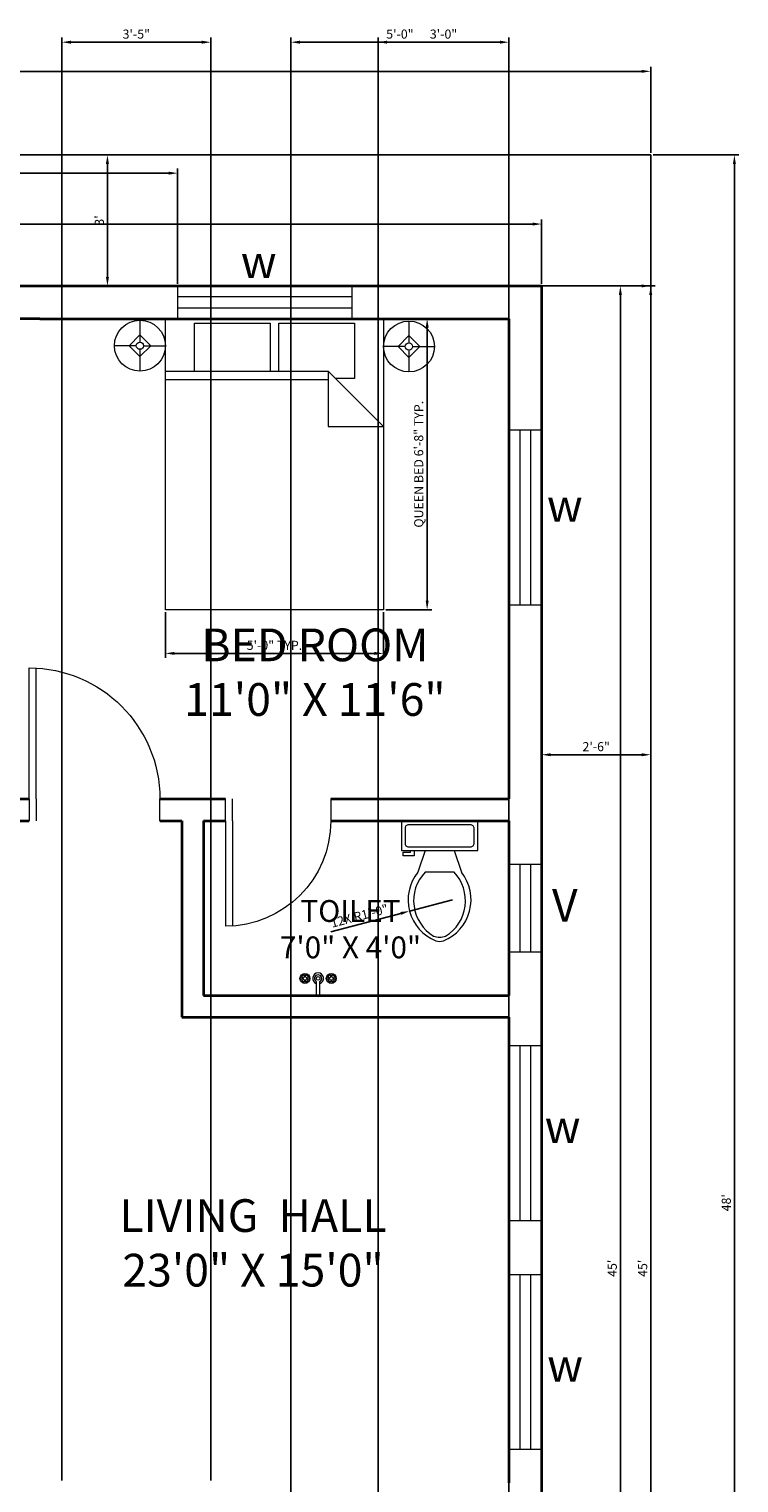
# Model space of a CAD drawing. Units: inches. Extents: x 2009 to 2890, y 2827 to 3504.
# Tile 3 of 6: x 2235 to 2430, y 3105 to 3504. Entities that reach past the tile are written whole.
import ezdxf

# ---------------------------------------------------------------- set-up
doc = ezdxf.new("R2010")
doc.units = ezdxf.units.IN
for name, color, linetype, lineweight in [('A-ANNO-DIMS', 2, 'Continuous', 18), ('A-ANNO-TEXT', 3, 'Continuous', 18), ('A-AREA-IDEN', 7, 'Continuous', 25), ('A-DOOR', 3, 'Continuous', 18), ('A-FLOR-FIXT', 9, 'Continuous', 18), ('A-FURN', 8, 'Continuous', 18), ('A-GLAZ', 4, 'Continuous', 18), ('A-WALL', 7, 'Continuous', 35), ('C-PROP', 8, 'Continuous', 25)]:
    doc.layers.add(name, color=color, linetype=linetype, lineweight=lineweight)
doc.styles.get("Standard").update_dxf_attribs({"font": 'arial.ttf'})
doc.dimstyles.new('ISO-25', dxfattribs={"dimtxt": 2.5, "dimasz": 2.5, "dimexe": 1.25, "dimexo": 0.625, "dimtad": 1, "dimdec": 0, "dimlunit": 3, "dimtxsty": 'Standard', "dimcen": 2.5, "dimadec": 0, "dimazin": 0, "dimtfac": 1, "dimtdec": 0, "dimtmove": 0, "dimatfit": 3, "dimfxl": 1, "dimarcsym": 0})

# ---------------------------------------------------------------- blocks, each defined once
blk = doc.blocks.new('Bed - Queen')
for p, q in [((0, -80.00003), (0, 0)), ((0, 0), (59.99999, 0)), ((59.99999, 0), (59.99999, -80.00003)), ((7.99999, -1.2), (28.79998, -1.2)), ((7.99999, -14.4), (7.99999, -1.2)), ((28.79998, -1.2), (28.79998, -14.4)), ((31.19999, -1.2), (51.99999, -1.2)), ((31.19999, -14.4), (31.19999, -1.2)), ((51.99999, -1.2), (51.99999, -16.4)), ((0, -14.4), (44.8, -14.4)), ((59.99999, -29.6), (44.8, -14.4)), ((44.8, -14.4), (44.8, -29.6)), ((44.8, -16.8), (0, -16.8)), ((51.99999, -16.4), (46.79936, -16.4)), ((44.8, -29.6), (59.99999, -29.6)), ((59.99999, -80.00003), (0, -80.00003))]:
    blk.add_line(p, q)
blk = doc.blocks.new('Lamp - Table')
for p, q in [((0, 7), (0, 1)), ((-1, 0), (-7, 0)), ((0, 3), (-3, 0)), ((-3, 0), (0, -3)), ((3, 0), (0, 3)), ((0, -3), (3, 0)), ((1, 0), (7, 0)), ((0, -1), (0, -7))]:
    blk.add_line(p, q)
for radius in [7, 1]:
    blk.add_circle((0, 0), radius)
blk = doc.blocks.new('Toilet - top')
for p, q in [((9.5, -6), (9.5, -2)), ((-10, -8.5), (-8, -8.5)), ((-10, -9.5), (-10, -8.5)), ((-7, -9.5), (-10, -9.5)), ((-8, -8.5), (-8, -8)), ((-7, -8), (-7, -9.5)), ((-4, -8), (-6, -14)), ((4, -8), (6, -14)), ((4, -14), (-4, -14))]:
    blk.add_line(p, q)
blk.add_lwpolyline([(10.5, -8), (10.5, 0), (-10.5, 0), (-10.5, -8)], close=True)
for points in [[(-9.5, -2), (-9.5, -6)], [(8.5, -1), (-8.5, -1)], [(-8.5, -7), (8.5, -7)]]:
    blk.add_lwpolyline(points)
for centre, radius, start, end in [((-8.62, -1.88), 0.884, 81.8699, 188.1301), ((8.62, -1.88), 0.884, 351.8699, 98.1301), ((-8.62, -6.12), 0.884, 171.8699, 278.1301), ((8.62, -6.12), 0.884, 261.8699, 8.1301), ((3.52, -21.58), 12.17, 141.4691, 247.9714), ((4.2, -21.82), 11.33, 136.3677, 238.9468), ((-3.52, -21.58), 12.17, 292.0284, 38.5307), ((-4.2, -21.82), 11.33, 301.053, 43.6321), ((0, -27.88), 4, 245.7318, 294.2682), ((0, -29), 4, 254.8605, 285.1395)]:
    blk.add_arc(centre, radius, start, end)
blk = doc.blocks.new('*D8')
at = {"layer": 'A-ANNO-DIMS', "color": 0, "lineweight": -2, "transparency": 16777216}
for p, q in [((2075.76, 3434.16), (2075.76, 3451.81)), ((2078.26, 3450.56), (2373.26, 3450.56)), ((2375.76, 3434.16), (2375.76, 3451.81))]:
    blk.add_line(p, q, dxfattribs=at)
at = {"layer": 'A-ANNO-DIMS', "color": 0, "transparency": 16777216}
for points in [[(2078.26, 3450.97), (2078.26, 3450.14), (2075.76, 3450.56)], [(2373.26, 3450.97), (2373.26, 3450.14), (2375.76, 3450.56)]]:
    blk.add_solid(points, dxfattribs=at)
at = {"layer": 'Defpoints', "color": 0, "transparency": 16777216}
for p in [(2375.76, 3450.56), (2075.76, 3433.54), (2375.76, 3433.54)]:
    blk.add_point(p, dxfattribs=at)
at = {"layer": 'A-ANNO-DIMS', "color": 0, "transparency": 16777216, "insert": (2225.76, 3452.46), "char_height": 2.5, "attachment_point": 5}
blk.add_mtext("25'", dxfattribs=at)
blk = doc.blocks.new('*D9')
at = {"layer": 'A-ANNO-DIMS', "color": 0, "lineweight": -2, "transparency": 16777216}
for p, q in [((2376.39, 3433.54), (2398.66, 3433.54)), ((2397.41, 3431.04), (2397.41, 2896.04)), ((2376.39, 2893.54), (2398.66, 2893.54))]:
    blk.add_line(p, q, dxfattribs=at)
at = {"layer": 'A-ANNO-DIMS', "color": 0, "transparency": 16777216}
for points in [[(2396.99, 3431.04), (2397.83, 3431.04), (2397.41, 3433.54)], [(2396.99, 2896.04), (2397.83, 2896.04), (2397.41, 2893.54)]]:
    blk.add_solid(points, dxfattribs=at)
at = {"layer": 'Defpoints', "color": 0, "transparency": 16777216}
for p in [(2375.76, 3433.54), (2375.76, 2893.54), (2397.41, 2893.54)]:
    blk.add_point(p, dxfattribs=at)
at = {"layer": 'A-ANNO-DIMS', "color": 0, "transparency": 16777216, "insert": (2395.51, 3163.54), "char_height": 2.5, "attachment_point": 5, "rotation": 90}
blk.add_mtext("45'", dxfattribs=at)
blk = doc.blocks.new('*D10')
at = {"layer": 'A-ANNO-DIMS', "color": 0, "lineweight": -2, "transparency": 16777216}
for p, q in [((2045.76, 3470.16), (2045.76, 3493.78)), ((2405.76, 3470.16), (2405.76, 3493.78)), ((2048.26, 3492.53), (2403.26, 3492.53))]:
    blk.add_line(p, q, dxfattribs=at)
at = {"layer": 'A-ANNO-DIMS', "color": 0, "transparency": 16777216}
for points in [[(2048.26, 3492.95), (2048.26, 3492.11), (2045.76, 3492.53)], [(2403.26, 3492.95), (2403.26, 3492.11), (2405.76, 3492.53)]]:
    blk.add_solid(points, dxfattribs=at)
at = {"layer": 'Defpoints', "color": 0, "transparency": 16777216}
for p in [(2405.76, 3492.53), (2045.76, 3469.54), (2405.76, 3469.54)]:
    blk.add_point(p, dxfattribs=at)
at = {"layer": 'A-ANNO-DIMS', "color": 0, "transparency": 16777216, "insert": (2225.76, 3494.43), "char_height": 2.5, "attachment_point": 5}
blk.add_mtext("30'", dxfattribs=at)
blk = doc.blocks.new('*D11')
at = {"layer": 'A-ANNO-DIMS', "color": 0, "lineweight": -2, "transparency": 16777216}
for p, q in [((2406.39, 3469.54), (2430.02, 3469.54)), ((2428.77, 3467.04), (2428.77, 2896.04)), ((2406.39, 2893.54), (2430.02, 2893.54))]:
    blk.add_line(p, q, dxfattribs=at)
at = {"layer": 'A-ANNO-DIMS', "color": 0, "transparency": 16777216}
for points in [[(2428.36, 3467.04), (2429.19, 3467.04), (2428.77, 3469.54)], [(2428.36, 2896.04), (2429.19, 2896.04), (2428.77, 2893.54)]]:
    blk.add_solid(points, dxfattribs=at)
at = {"layer": 'Defpoints', "color": 0, "transparency": 16777216}
for p in [(2405.76, 3469.54), (2405.76, 2893.54), (2428.77, 2893.54)]:
    blk.add_point(p, dxfattribs=at)
at = {"layer": 'A-ANNO-DIMS', "color": 0, "transparency": 16777216, "insert": (2426.87, 3181.54), "char_height": 2.5, "attachment_point": 5, "rotation": 90}
blk.add_mtext("48'", dxfattribs=at)
blk = doc.blocks.new('Faucet - Bathroom top')
for p, q in [((-4.107, 0.125), (-4.375, 0.125)), ((-3.75, 0.4788), (-3.75, 0.75)), ((-3.5, 0.482), (-3.5, 0.75)), ((-3.1461, 0.125), (-2.875, 0.125)), ((3.143, 0.125), (2.875, 0.125)), ((3.5, 0.4788), (3.5, 0.75)), ((3.75, 0.482), (3.75, 0.75)), ((4.1039, 0.125), (4.375, 0.125)), ((-4.1039, -0.125), (-4.375, -0.125)), ((-3.75, -0.4821), (-3.75, -0.75)), ((-3.5, -0.4789), (-3.5, -0.75)), ((-3.143, -0.125), (-2.875, -0.125)), ((-0.5, -0.8639), (-0.5, -4.5)), ((0.5, -4.5), (0.5, -0.8631)), ((3.1461, -0.125), (2.875, -0.125)), ((3.5, -0.4821), (3.5, -0.75)), ((3.75, -0.4789), (3.75, -0.75)), ((4.107, -0.125), (4.375, -0.125))]:
    blk.add_line(p, q)
for centre, radius in [((-3.625, 0), 1.375), ((-4.625, 0), 0.2795), ((-3.625, 0), 0.5), ((-3.625, 1), 0.2795), ((-2.625, 0), 0.2795), ((0, 0), 0.5), ((3.625, 0), 1.375), ((2.625, 0), 0.2795), ((3.625, 0), 0.5), ((3.625, 1), 0.2795), ((4.625, 0), 0.2795), ((-3.625, -1), 0.2795), ((3.625, -1), 0.2795)]:
    blk.add_circle(centre, radius)
for centre, radius, start, end in [((-3.625, 0), 1, 105.2407, 164.2093), ((-3.625, 0), 1, 16.44125, 74.07887), ((0, 0), 1.5, 289.6514, 250.3603), ((0, 0), 1, 300.3431, 239.7554), ((3.625, 0), 1, 106.12, 164.0884), ((3.625, 0), 1, 16.23422, 73.90469), ((-3.625, 0), 1, 196.2342, 253.9047), ((-3.625, 0), 1, 286.12, 344.0884), ((3.625, 0), 1, 196.4413, 254.0789), ((3.625, 0), 1, 285.2407, 344.2093), ((0, -4.5), 0.5, 180, 0)]:
    blk.add_arc(centre, radius, start, end)
blk = doc.blocks.new('*D16')
at = {"layer": 'A-ANNO-DIMS', "color": 0, "lineweight": -2, "transparency": 16777216}
for p, q in [((2045.76, 3468.91), (2045.76, 3432.29)), ((2405.76, 3468.91), (2405.76, 3432.29)), ((2403.26, 3433.54), (2048.26, 3433.54))]:
    blk.add_line(p, q, dxfattribs=at)
at = {"layer": 'A-ANNO-DIMS', "color": 0, "transparency": 16777216}
for points in [[(2048.26, 3433.96), (2048.26, 3433.12), (2045.76, 3433.54)], [(2403.26, 3433.96), (2403.26, 3433.12), (2405.76, 3433.54)]]:
    blk.add_solid(points, dxfattribs=at)
at = {"layer": 'Defpoints', "color": 0, "transparency": 16777216}
for p in [(2045.76, 3469.54), (2405.76, 3469.54), (2045.76, 3433.54)]:
    blk.add_point(p, dxfattribs=at)
at = {"layer": 'A-ANNO-DIMS', "color": 0, "transparency": 16777216, "insert": (2225.76, 3435.44), "char_height": 2.5, "attachment_point": 5}
blk.add_mtext("30'", dxfattribs=at)
blk = doc.blocks.new('*D17')
at = {"layer": 'A-ANNO-DIMS', "color": 0, "lineweight": -2, "transparency": 16777216}
for p, q in [((2257.96, 3469.54), (2255.07, 3469.54)), ((2256.32, 3467.04), (2256.32, 3436.04)), ((2257.96, 3433.54), (2255.07, 3433.54))]:
    blk.add_line(p, q, dxfattribs=at)
at = {"layer": 'A-ANNO-DIMS', "color": 0, "transparency": 16777216}
for points in [[(2255.9, 3467.04), (2256.74, 3467.04), (2256.32, 3469.54)], [(2255.9, 3436.04), (2256.74, 3436.04), (2256.32, 3433.54)]]:
    blk.add_solid(points, dxfattribs=at)
at = {"layer": 'Defpoints', "color": 0, "transparency": 16777216}
for p in [(2258.58, 3469.54), (2256.32, 3433.54), (2258.58, 3433.54)]:
    blk.add_point(p, dxfattribs=at)
at = {"layer": 'A-ANNO-DIMS', "color": 0, "transparency": 16777216, "insert": (2254.42, 3451.54), "char_height": 2.5, "attachment_point": 5, "rotation": 90}
blk.add_mtext("3'", dxfattribs=at)
blk = doc.blocks.new('*D18')
at = {"layer": 'A-ANNO-DIMS', "color": 0, "lineweight": -2, "transparency": 16777216}
for p, q in [((2376.39, 3433.54), (2407.01, 3433.54)), ((2405.76, 3431.04), (2405.76, 2896.04)), ((2376.39, 2893.54), (2407.01, 2893.54))]:
    blk.add_line(p, q, dxfattribs=at)
at = {"layer": 'A-ANNO-DIMS', "color": 0, "transparency": 16777216}
for points in [[(2405.35, 3431.04), (2406.18, 3431.04), (2405.76, 3433.54)], [(2405.35, 2896.04), (2406.18, 2896.04), (2405.76, 2893.54)]]:
    blk.add_solid(points, dxfattribs=at)
at = {"layer": 'Defpoints', "color": 0, "transparency": 16777216}
for p in [(2375.76, 3433.54), (2375.76, 2893.54), (2405.76, 2893.54)]:
    blk.add_point(p, dxfattribs=at)
at = {"layer": 'A-ANNO-DIMS', "color": 0, "transparency": 16777216, "insert": (2403.87, 3163.54), "char_height": 2.5, "attachment_point": 5, "rotation": 90}
blk.add_mtext("45'", dxfattribs=at)
blk = doc.blocks.new('*D19')
at = {"layer": 'A-ANNO-DIMS', "color": 0, "lineweight": -2, "transparency": 16777216}
for p, q in [((2376.39, 3433.54), (2407.01, 3433.54)), ((2405.76, 3431.04), (2405.76, 2896.04)), ((2376.39, 2893.54), (2407.01, 2893.54))]:
    blk.add_line(p, q, dxfattribs=at)
at = {"layer": 'A-ANNO-DIMS', "color": 0, "transparency": 16777216}
for points in [[(2405.35, 3431.04), (2406.18, 3431.04), (2405.76, 3433.54)], [(2405.35, 2896.04), (2406.18, 2896.04), (2405.76, 2893.54)]]:
    blk.add_solid(points, dxfattribs=at)
at = {"layer": 'Defpoints', "color": 0, "transparency": 16777216}
for p in [(2375.76, 3433.54), (2375.76, 2893.54), (2405.76, 2893.54)]:
    blk.add_point(p, dxfattribs=at)
at = {"layer": 'A-ANNO-DIMS', "color": 0, "transparency": 16777216, "insert": (2403.87, 3163.54), "char_height": 2.5, "attachment_point": 5, "rotation": 90}
blk.add_mtext("45'", dxfattribs=at)
blk = doc.blocks.new('*D20')
at = {"layer": 'A-ANNO-DIMS', "color": 0, "lineweight": -2, "transparency": 16777216}
for p, q in [((2375.76, 3320.11), (2375.76, 3303.44)), ((2405.76, 3320.11), (2405.76, 3303.44)), ((2378.26, 3304.69), (2403.26, 3304.69))]:
    blk.add_line(p, q, dxfattribs=at)
at = {"layer": 'A-ANNO-DIMS', "color": 0, "transparency": 16777216}
for points in [[(2378.26, 3305.11), (2378.26, 3304.27), (2375.76, 3304.69)], [(2403.26, 3305.11), (2403.26, 3304.27), (2405.76, 3304.69)]]:
    blk.add_solid(points, dxfattribs=at)
at = {"layer": 'Defpoints', "color": 0, "transparency": 16777216}
for p in [(2375.76, 3320.74), (2405.76, 3320.74), (2405.76, 3304.69)]:
    blk.add_point(p, dxfattribs=at)
at = {"layer": 'A-ANNO-DIMS', "color": 0, "transparency": 16777216, "insert": (2390.76, 3306.59), "char_height": 2.5, "attachment_point": 5}
blk.add_mtext('2\'-6"', dxfattribs=at)
blk = doc.blocks.new('WIN-48IN')
for p, q in [((0, 48), (0, 0)), ((9, 48), (0, 48)), ((3, 48), (3, 0)), ((6, 0), (6, 48)), ((9, 0), (9, 48)), ((0, 0), (9, 0))]:
    blk.add_line(p, q)
blk = doc.blocks.new('VENT-24IN')
for p, q in [((0, 24), (0, 0)), ((9, 24), (0, 24)), ((3, 24), (3, 0)), ((6, 0), (6, 24)), ((9, 0), (9, 24)), ((0, 0), (9, 0))]:
    blk.add_line(p, q)
blk = doc.blocks.new('DOOR-29IN')
for p, q in [((0, 35), (0, 29)), ((27, 29), (27, 35)), ((29, 29), (29, 35)), ((27, 29), (27, 0)), ((29, 29), (29, 0))]:
    blk.add_line(p, q)
blk.add_arc((29, 29), 29, 180, 270)
blk = doc.blocks.new('DOOR-36IN')
for p, q in [((34, 6), (34, 42)), ((36, 6), (36, 42)), ((0, 0), (0, 6)), ((34, 6), (34, 0)), ((36, 6), (36, 0))]:
    blk.add_line(p, q)
blk.add_arc((36, 6), 36, 90, 180)
blk = doc.blocks.new('*D43')
at = {"layer": 'A-ANNO-DIMS', "color": 0, "lineweight": -2, "transparency": 16777216}
for p, q in [((2332.89, 3424.54), (2345.51, 3424.54)), ((2344.26, 3347.04), (2344.26, 3422.04)), ((2332.89, 3344.54), (2345.51, 3344.54))]:
    blk.add_line(p, q, dxfattribs=at)
at = {"layer": 'A-ANNO-DIMS', "color": 0, "transparency": 16777216}
for points in [[(2343.85, 3422.04), (2344.68, 3422.04), (2344.26, 3424.54)], [(2343.85, 3347.04), (2344.68, 3347.04), (2344.26, 3344.54)]]:
    blk.add_solid(points, dxfattribs=at)
at = {"layer": 'Defpoints', "color": 0, "transparency": 16777216}
for p in [(2332.26, 3424.54), (2344.26, 3424.54), (2332.26, 3344.54)]:
    blk.add_point(p, dxfattribs=at)
at = {"layer": 'A-ANNO-DIMS', "color": 0, "transparency": 16777216, "insert": (2342.27, 3384.54), "char_height": 2.5, "attachment_point": 5, "rotation": 90}
blk.add_mtext('QUEEN BED 6\'-8" TYP.', dxfattribs=at)
blk = doc.blocks.new('*D44')
at = {"layer": 'A-ANNO-DIMS', "color": 0, "lineweight": -2, "transparency": 16777216}
for p, q in [((2272.26, 3343.91), (2272.26, 3331.29)), ((2332.26, 3343.91), (2332.26, 3331.29)), ((2274.76, 3332.54), (2329.76, 3332.54))]:
    blk.add_line(p, q, dxfattribs=at)
at = {"layer": 'A-ANNO-DIMS', "color": 0, "transparency": 16777216}
for points in [[(2274.76, 3332.96), (2274.76, 3332.12), (2272.26, 3332.54)], [(2329.76, 3332.96), (2329.76, 3332.12), (2332.26, 3332.54)]]:
    blk.add_solid(points, dxfattribs=at)
at = {"layer": 'Defpoints', "color": 0, "transparency": 16777216}
for p in [(2272.26, 3344.54), (2332.26, 3344.54), (2332.26, 3332.54)]:
    blk.add_point(p, dxfattribs=at)
at = {"layer": 'A-ANNO-DIMS', "color": 0, "transparency": 16777216, "insert": (2302.26, 3334.44), "char_height": 2.5, "attachment_point": 5}
blk.add_mtext('5\'-0" TYP.', dxfattribs=at)
blk = doc.blocks.new('*D66')
at = {"layer": 'A-ANNO-DIMS', "color": 0, "lineweight": -2, "transparency": 16777216}
for p, q in [((2330.76, 3011.16), (2330.76, 3501.79)), ((2366.76, 3011.16), (2366.76, 3501.79)), ((2333.26, 3500.54), (2364.26, 3500.54))]:
    blk.add_line(p, q, dxfattribs=at)
at = {"layer": 'A-ANNO-DIMS', "color": 0, "transparency": 16777216}
for points in [[(2333.26, 3500.96), (2333.26, 3500.12), (2330.76, 3500.54)], [(2364.26, 3500.96), (2364.26, 3500.12), (2366.76, 3500.54)]]:
    blk.add_solid(points, dxfattribs=at)
at = {"layer": 'Defpoints', "color": 0, "transparency": 16777216}
for p in [(2366.76, 3500.54), (2330.76, 3010.54), (2366.76, 3010.54)]:
    blk.add_point(p, dxfattribs=at)
at = {"layer": 'A-ANNO-DIMS', "color": 0, "transparency": 16777216, "insert": (2348.76, 3502.44), "char_height": 2.5, "attachment_point": 5}
blk.add_mtext('3\'-0"', dxfattribs=at)
blk = doc.blocks.new('*D68')
at = {"layer": 'A-ANNO-DIMS', "color": 0, "lineweight": -2, "transparency": 16777216}
for p, q in [((2306.76, 3048.16), (2306.76, 3501.79)), ((2366.76, 3048.16), (2366.76, 3501.79)), ((2309.26, 3500.54), (2364.26, 3500.54))]:
    blk.add_line(p, q, dxfattribs=at)
at = {"layer": 'A-ANNO-DIMS', "color": 0, "transparency": 16777216}
for points in [[(2309.26, 3500.96), (2309.26, 3500.12), (2306.76, 3500.54)], [(2364.26, 3500.96), (2364.26, 3500.12), (2366.76, 3500.54)]]:
    blk.add_solid(points, dxfattribs=at)
at = {"layer": 'Defpoints', "color": 0, "transparency": 16777216}
for p in [(2366.76, 3500.54), (2306.76, 3047.54), (2366.76, 3047.54)]:
    blk.add_point(p, dxfattribs=at)
at = {"layer": 'A-ANNO-DIMS', "color": 0, "transparency": 16777216, "insert": (2336.76, 3502.44), "char_height": 2.5, "attachment_point": 5}
blk.add_mtext('5\'-0"', dxfattribs=at)
blk = doc.blocks.new('*D75')
at = {"layer": 'A-ANNO-DIMS', "color": 0, "lineweight": -2, "transparency": 16777216}
for p, q in [((2243.76, 3105.16), (2243.76, 3501.79)), ((2284.76, 3105.16), (2284.76, 3501.79)), ((2246.26, 3500.54), (2282.26, 3500.54))]:
    blk.add_line(p, q, dxfattribs=at)
at = {"layer": 'A-ANNO-DIMS', "color": 0, "transparency": 16777216}
for points in [[(2246.26, 3500.96), (2246.26, 3500.12), (2243.76, 3500.54)], [(2282.26, 3500.96), (2282.26, 3500.12), (2284.76, 3500.54)]]:
    blk.add_solid(points, dxfattribs=at)
at = {"layer": 'Defpoints', "color": 0, "transparency": 16777216}
for p in [(2284.76, 3500.54), (2243.76, 3104.54), (2284.76, 3104.54)]:
    blk.add_point(p, dxfattribs=at)
at = {"layer": 'A-ANNO-DIMS', "color": 0, "transparency": 16777216, "insert": (2264.26, 3502.44), "char_height": 2.5, "attachment_point": 5}
blk.add_mtext('3\'-5"', dxfattribs=at)
blk = doc.blocks.new('*D77')
at = {"layer": 'A-ANNO-DIMS', "color": 0, "lineweight": -2, "transparency": 16777216}
for p, q in [((2130.69, 3434.16), (2130.69, 3465.79)), ((2275.62, 3434.16), (2275.62, 3465.79)), ((2133.19, 3464.54), (2273.12, 3464.54))]:
    blk.add_line(p, q, dxfattribs=at)
at = {"layer": 'A-ANNO-DIMS', "color": 0, "transparency": 16777216}
for points in [[(2133.19, 3464.96), (2133.19, 3464.12), (2130.69, 3464.54)], [(2273.12, 3464.96), (2273.12, 3464.12), (2275.62, 3464.54)]]:
    blk.add_solid(points, dxfattribs=at)
at = {"layer": 'Defpoints', "color": 0, "transparency": 16777216}
for p in [(2275.62, 3464.54), (2130.69, 3433.54), (2275.62, 3433.54)]:
    blk.add_point(p, dxfattribs=at)
at = {"layer": 'A-ANNO-DIMS', "color": 0, "transparency": 16777216, "insert": (2203.16, 3466.42), "char_height": 2.5, "attachment_point": 5}
blk.add_mtext('12\'-1"', dxfattribs=at)
blk = doc.blocks.new('*D91')
at = {"layer": 'A-ANNO-DIMS', "color": 0, "lineweight": -2, "transparency": 16777216}
for p, q in [((2351.2, 3264.81), (2339.43, 3261.71)), ((2317.8, 3256.03), (2337.01, 3261.08))]:
    blk.add_line(p, q, dxfattribs=at)
at = {"layer": 'A-ANNO-DIMS', "color": 0, "transparency": 16777216}
blk.add_solid([(2336.91, 3261.48), (2337.12, 3260.68), (2339.43, 3261.71)], dxfattribs=at)
at = {"layer": 'Defpoints', "color": 0, "transparency": 16777216}
for p in [(2351.2, 3264.81), (2339.43, 3261.71)]:
    blk.add_point(p, dxfattribs=at)
at = {"layer": 'A-ANNO-DIMS', "color": 0, "transparency": 16777216, "insert": (2325.71, 3260.08), "char_height": 2.5, "attachment_point": 5, "rotation": 14.7219}
blk.add_mtext('12X R1\'-0"', dxfattribs=at)

msp = doc.modelspace()

# ---------------------------------------------------------------- linework, layer by layer
at = {"layer": 'A-WALL'}
for p, q in [((2075.76, 3433.54), (2375.76, 3433.54)), ((2375.76, 3433.54), (2375.76, 2893.54)), ((2237.76, 3424.54), (2228.76, 3424.54)), ((2237.76, 3424.54), (2366.76, 3424.54)), ((2366.76, 3424.54), (2366.76, 3292.54)), ((2228.76, 3292.54), (2234.76, 3292.54)), ((2228.76, 3292.54), (2234.76, 3292.54)), ((2270.76, 3292.54), (2288.76, 3292.54)), ((2317.76, 3292.54), (2366.76, 3292.54)), ((2216.76, 3286.54), (2234.76, 3286.54)), ((2270.76, 3286.54), (2276.76, 3286.54)), ((2276.76, 3286.54), (2276.76, 3238.54)), ((2282.76, 3286.54), (2282.76, 3238.54)), ((2282.76, 3286.54), (2288.76, 3286.54)), ((2282.76, 3286.54), (2288.76, 3286.54)), ((2317.76, 3286.54), (2366.76, 3286.54)), ((2366.76, 3286.54), (2366.76, 3238.54)), ((2276.76, 3238.54), (2276.76, 3232.54)), ((2282.76, 3238.54), (2366.76, 3238.54)), ((2276.76, 3232.54), (2366.76, 3232.54)), ((2366.76, 3232.54), (2366.76, 3104.54))]:
    msp.add_line(p, q, dxfattribs=at)
at = {"layer": 'C-PROP'}
for p, q in [((2045.76, 3469.54), (2405.76, 3469.54)), ((2405.76, 3469.54), (2045.76, 3469.54)), ((2045.76, 3469.54), (2405.76, 3469.54)), ((2405.76, 3469.54), (2045.76, 3469.54)), ((2075.76, 3469.54), (2375.76, 3469.54)), ((2375.76, 3469.54), (2405.76, 3469.54)), ((2405.76, 3433.54), (2405.76, 3469.54)), ((2405.76, 3433.54), (2405.76, 2893.54))]:
    msp.add_line(p, q, dxfattribs=at)

# ---------------------------------------------------------------- block references
at = {"layer": 'A-DOOR', "extrusion": (0, 0, -1), "zscale": -1}
for name, p in [('DOOR-36IN', (-2270.76, 3286.54)), ('DOOR-29IN', (-2317.76, 3257.54))]:
    msp.add_blockref(name, p, dxfattribs=at)
at = {"layer": 'A-FLOR-FIXT'}
for name, p in [('Toilet - top', (2347.68, 3286.39)), ('Faucet - Bathroom top', (2314.28, 3243.2))]:
    msp.add_blockref(name, p, dxfattribs=at)
at = {"layer": 'A-FURN'}
for name, p in [('Lamp - Table', (2265.26, 3417.12)), ('Bed - Queen', (2272.26, 3424.54)), ('Lamp - Table', (2339.26, 3416.89))]:
    msp.add_blockref(name, p, dxfattribs=at)
at = {"layer": 'A-GLAZ', "rotation": 270.0000000000037}
msp.add_blockref('WIN-48IN', (2275.62, 3433.54), dxfattribs=at)
at = {"layer": 'A-GLAZ'}
for name, p in [('WIN-48IN', (2366.76, 3345.92)), ('VENT-24IN', (2366.76, 3250.54)), ('WIN-48IN', (2366.76, 3176.67)), ('WIN-48IN', (2366.76, 3113.78))]:
    msp.add_blockref(name, p, dxfattribs=at)

# ---------------------------------------------------------------- texts
at = {"layer": 'A-ANNO-TEXT', "char_height": 9, "attachment_point": 1}
for s, width, insert in [('\\pxqc;w', 53.6341, (2271.11, 3444.68)), ('\\pxqc;w', 53.6341, (2355.3, 3377.71)), ('\\pxqc;V', 57.7621, (2353.24, 3267.82)), ('\\pxqc;w', 53.6341, (2354.7, 3207)), ('\\pxqc;w', 53.6341, (2355.39, 3141.4))]:
    msp.add_mtext_dynamic_manual_height_columns(s, width=width, gutter_width=12.5, heights=[0], dxfattribs=dict(at, insert=insert))
at = {"layer": 'A-AREA-IDEN', "attachment_point": 1}
for s, width, insert, char_height in [('\\pxqc;BED ROOM\\P11\'0" X 11\'6" ', 85.3364, (2270.72, 3339.38), 9), ('\\pxqc;TOILET\\P7\'0" X 4\'0"', 53.3807, (2296.48, 3264.74), 6), ('\\pxqc;LIVING  HALL\\P23\'0" X 15\'0" ', 102.762, (2244.97, 3182.52), 9)]:
    msp.add_mtext_dynamic_manual_height_columns(s, width=width, gutter_width=12.5, heights=[0], dxfattribs=dict(at, insert=insert, char_height=char_height))

# ---------------------------------------------------------------- dimensions: what is measured, and where the dimension line sits
at = {"layer": 'A-ANNO-DIMS'}
for base, p1, p2, override, picture, middle in [((2284.76, 3500.54), (2243.76, 3104.54), (2284.76, 3104.54), {"dimdec": 1, "dimlfac": 1, "dimrnd": 0, "dimzin": 1, "dimdsep": 46, "dimlunit": 4, "dimfrac": 2}, '*D75', (2264.26, 3502.44)), ((2366.76, 3500.54), (2306.76, 3047.54), (2366.76, 3047.54), {"dimdec": 1, "dimlfac": 1, "dimrnd": 0, "dimzin": 1, "dimdsep": 46, "dimlunit": 4, "dimfrac": 2}, '*D68', (2336.76, 3502.44)), ((2366.76, 3500.54), (2330.76, 3010.54), (2366.76, 3010.54), {"dimdec": 1, "dimlfac": 1, "dimrnd": 0, "dimzin": 1, "dimdsep": 46, "dimlunit": 4, "dimfrac": 2}, '*D66', (2348.76, 3502.44)), ((2405.76, 3492.53), (2045.76, 3469.54), (2405.76, 3469.54), {"dimclrd": 0, "dimclre": 0, "dimclrt": 0}, '*D10', (2225.76, 3494.43)), ((2045.76, 3433.54), (2405.76, 3469.54), (2045.76, 3469.54), {"dimclrd": 0, "dimclre": 0, "dimclrt": 0}, '*D16', (2225.76, 3435.44)), ((2275.62, 3464.54), (2130.69, 3433.54), (2275.62, 3433.54), {"dimdec": 1, "dimlfac": 1, "dimrnd": 0, "dimzin": 1, "dimdsep": 46, "dimlunit": 4, "dimfrac": 2}, '*D77', (2203.16, 3466.42)), ((2375.76, 3450.56), (2075.76, 3433.54), (2375.76, 3433.54), {"dimclrd": 0, "dimclre": 0, "dimclrt": 0}, '*D8', (2225.76, 3452.46)), ((2405.76, 3304.69), (2375.76, 3320.74), (2405.76, 3320.74), {"dimclrd": 0, "dimclre": 0, "dimclrt": 0}, '*D20', (2390.76, 3306.59))]:
    dim = msp.add_linear_dim(base=base, p1=p1, p2=p2, dimstyle='ISO-25', override=override, dxfattribs=at)
    dim.commit()
    dim.dimension.update_dxf_attribs({"geometry": picture, "text_midpoint": middle})
for base, p1, p2, picture, middle in [((2256.32, 3433.54), (2258.58, 3469.54), (2258.58, 3433.54), '*D17', (2254.42, 3451.54)), ((2428.77, 2893.54), (2405.76, 3469.54), (2405.76, 2893.54), '*D11', (2426.87, 3181.54)), ((2397.41, 2893.54), (2375.76, 3433.54), (2375.76, 2893.54), '*D9', (2395.51, 3163.54)), ((2405.76, 2893.54), (2375.76, 3433.54), (2375.76, 2893.54), '*D18', (2403.87, 3163.54)), ((2405.76, 2893.54), (2375.76, 3433.54), (2375.76, 2893.54), '*D19', (2403.87, 3163.54))]:
    dim = msp.add_linear_dim(base=base, p1=p1, p2=p2, angle=90, dimstyle='ISO-25', override={"dimclrd": 0, "dimclre": 0, "dimclrt": 0}, dxfattribs=at)
    dim.commit()
    dim.dimension.update_dxf_attribs({"geometry": picture, "text_midpoint": middle})
dim = msp.add_linear_dim(base=(2344.26, 3424.54), p1=(2332.26, 3344.54), p2=(2332.26, 3424.54), angle=90, text='QUEEN BED <> TYP.', dimstyle='ISO-25', override={"dimdec": 1, "dimlfac": 1, "dimrnd": 0, "dimzin": 1, "dimdsep": 46, "dimlunit": 4, "dimfrac": 2}, dxfattribs=at)
dim.commit()
dim.dimension.update_dxf_attribs({"geometry": '*D43', "text_midpoint": (2342.27, 3384.54)})
dim = msp.add_linear_dim(base=(2332.26, 3332.54), p1=(2272.26, 3344.54), p2=(2332.26, 3344.54), text='<> TYP.', dimstyle='ISO-25', override={"dimdec": 1, "dimlfac": 1, "dimrnd": 0, "dimzin": 1, "dimdsep": 46, "dimlunit": 4, "dimfrac": 2}, dxfattribs=at)
dim.commit()
dim.dimension.update_dxf_attribs({"geometry": '*D44', "text_midpoint": (2302.26, 3334.44)})
dim = msp.add_radius_dim(center=(2351.2, 3264.81), mpoint=(2339.43, 3261.71), text='12X <>', dimstyle='ISO-25', override={"dimdec": 1, "dimlfac": 1, "dimrnd": 0, "dimzin": 1, "dimdsep": 46, "dimlunit": 4, "dimfrac": 2}, dxfattribs=at)
dim.commit()
dim.dimension.update_dxf_attribs({"geometry": '*D91', "text_midpoint": (2325.71, 3260.08)})

doc.saveas('drawing.dxf')
